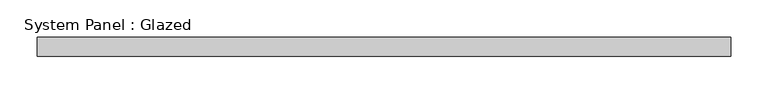
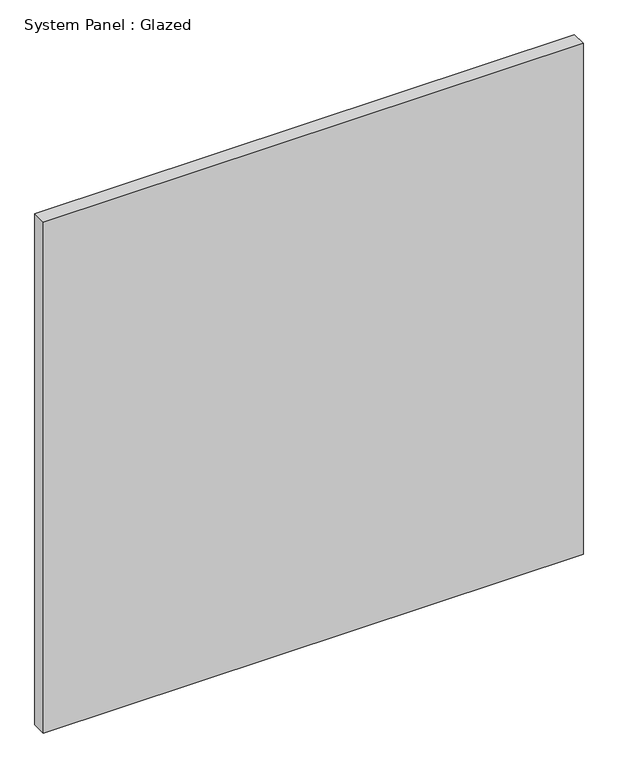
"""IFC4 building model written with IfcOpenShell, lengths in millimetres: plate geometry, System Panel : Glazed."""

from ifc_helpers import new_model, si_unit, origin, origin_with_axes, place, context, project, spatial, polyline, outline, extrude, source, transform, mapped, element, save


def system_panel_glazed_7f04015b(model_context):
    return source(origin(), model_context, "Body", "SweptSolid", [
        extrude(outline(polyline([(463.5500002, 19.05), (-463.5500002, 19.05), (-463.5500002, 44.45), (463.5500002, 44.45), (463.5500002, 19.05)])), origin_with_axes(), (0.0, 0.0, 1.0), 927.1),
    ])


if __name__ == "__main__":
    model = new_model("IFC4")
    model_context = context("Model", 3, world=origin())
    ifc_project = project(units=[si_unit("LENGTHUNIT", "METRE", prefix="MILLI")], contexts=[model_context])
    site = spatial("IfcSite", under=ifc_project)
    building = spatial("IfcBuilding", under=site)
    placement = place(None, origin())
    system_panel_glazed_shape = system_panel_glazed_7f04015b(model_context)
    element("IfcPlate", 1, ObjectType="System Panel : Glazed", at=placement, inside=building, context=model_context, shape_type="MappedRepresentation", body=[
        mapped(system_panel_glazed_shape, transform((0.0, 0.0, 0.0), x_axis=(1.0, 0.0, 0.0), y_axis=(0.0, 1.0, 0.0), z_axis=(0.0, 0.0, 1.0))),
    ])
    save(model, "model.ifc")

# Revit data of these elements
# Type "System Panel : Glazed"
#   Construction Type Id = "GSP4R"
#   Analytic Construction = "1/8 in Pilkington single glazing"
#   Visual Light Transmittance = 0.9
#   Solar Heat Gain Coefficient = 0.86
#   Heat Transfer Coefficient (U) = 1.18115 BTU/(h·ft²·°F)
#   Define Thermal Properties by = 1
# Element 1 (IfcPlate, "System Panel : Glazed")
#   Materials on its faces: "Glass"
# Materials
#   "Glass": class "Glass", colour RGB 0 128 192, transparency 0.75, Description = "Soda Lime Glass", Cost = 0
